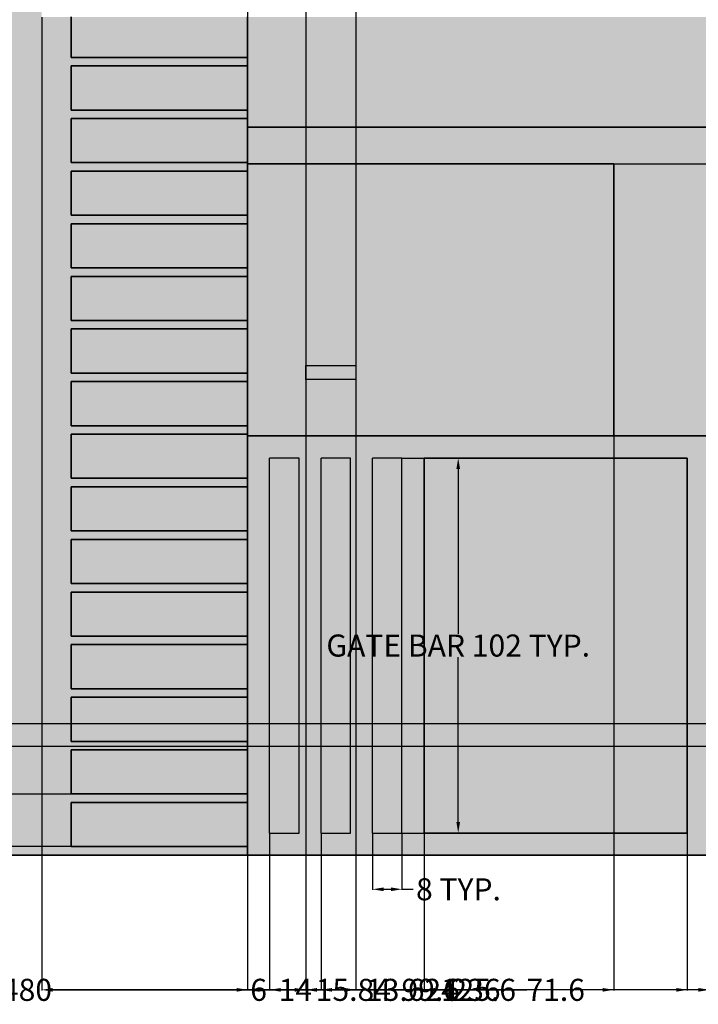
# Model space of a CAD drawing. Units: inches. Extents: x 126 to 726, y 86 to 888.
# Tile 4 of 13: x 424 to 609, y 86 to 354. Entities that reach past the tile are written whole.
import ezdxf

# ---------------------------------------------------------------- set-up
doc = ezdxf.new("R2010")
doc.units = ezdxf.units.IN
doc.header["$MEASUREMENT"] = 0
for name, color, linetype, lineweight in [('A-ANNO-DIMS', 2, 'Continuous', 18), ('A-DOOR', 3, 'Continuous', 25), ('A-ELEV', 7, 'Continuous', 35), ('A-ELEV-GATE', 7, 'Continuous', 25), ('A-ELEV-PATT', 8, 'Continuous', 13)]:
    doc.layers.add(name, color=color, linetype=linetype, lineweight=lineweight)
doc.styles.get("Standard").update_dxf_attribs({"font": 'arial.ttf'})
doc.dimstyles.get("Standard").update_dxf_attribs({"dimtxt": 6, "dimasz": 3, "dimexe": 0.18, "dimexo": 0.0625, "dimgap": 0.09, "dimtad": 0, "dimtih": 1, "dimtoh": 1, "dimdec": 0, "dimzin": 0, "dimdsep": 46, "dimlunit": 3, "dimtxsty": 'Standard', "dimcen": 0.09, "dimadec": 0, "dimazin": 0, "dimtfac": 1, "dimtdec": 0, "dimtofl": 0, "dimtmove": 0, "dimatfit": 3, "dimfxl": 1, "dimtolj": 1, "dimtzin": 0, "dimarcsym": 0})

# ---------------------------------------------------------------- blocks, each defined once
blk = doc.blocks.new('FACADE-STRIP')
for p, q in [((0, 0), (0, 12)), ((0, 12), (48, 12)), ((0, 0), (48, 0))]:
    blk.add_line(p, q)
blk = doc.blocks.new('GATE-BAR')
for p, q in [((0, 0), (0, 102)), ((8, 102), (0, 102)), ((8, 0), (8, 102)), ((0, 0), (8, 0))]:
    blk.add_line(p, q)
blk = doc.blocks.new('*D7')
at = {"layer": 'A-ANNO-DIMS', "color": 0, "lineweight": -2, "transparency": 16777216}
for p, q in [((528.04, 235.04), (543.45, 235.04)), ((543.27, 232.04), (543.27, 187.23)), ((543.27, 136.04), (543.27, 180.85)), ((528.04, 133.04), (543.45, 133.04))]:
    blk.add_line(p, q, dxfattribs=at)
at = {"layer": 'A-ANNO-DIMS', "color": 0, "transparency": 16777216}
for points in [[(542.77, 232.04), (543.77, 232.04), (543.27, 235.04)], [(542.77, 136.04), (543.77, 136.04), (543.27, 133.04)]]:
    blk.add_solid(points, dxfattribs=at)
at = {"layer": 'Defpoints', "color": 0, "transparency": 16777216}
for p in [(527.97, 235.04), (543.27, 235.04), (527.97, 133.04)]:
    blk.add_point(p, dxfattribs=at)
at = {"layer": 'A-ANNO-DIMS', "color": 0, "transparency": 16777216, "insert": (543.27, 184.04), "char_height": 6, "attachment_point": 5}
blk.add_mtext('\\A1;GATE BAR 102 TYP.', dxfattribs=at)
blk = doc.blocks.new('*D8')
at = {"layer": 'A-ANNO-DIMS', "color": 0, "lineweight": -2, "transparency": 16777216}
for p, q in [((519.97, 132.98), (519.97, 117.56)), ((527.97, 132.98), (527.97, 117.56)), ((522.97, 117.74), (524.97, 117.74)), ((527.97, 117.74), (530.97, 117.74))]:
    blk.add_line(p, q, dxfattribs=at)
at = {"layer": 'A-ANNO-DIMS', "color": 0, "transparency": 16777216}
for points in [[(522.97, 118.24), (522.97, 117.24), (519.97, 117.74)], [(524.97, 118.24), (524.97, 117.24), (527.97, 117.74)]]:
    blk.add_solid(points, dxfattribs=at)
at = {"layer": 'Defpoints', "color": 0, "transparency": 16777216}
for p in [(519.97, 133.04), (527.97, 133.04), (527.97, 117.74)]:
    blk.add_point(p, dxfattribs=at)
at = {"layer": 'A-ANNO-DIMS', "color": 0, "transparency": 16777216, "insert": (543.34, 117.74), "char_height": 6, "attachment_point": 5}
blk.add_mtext('\\A1;8 TYP.', dxfattribs=at)
blk = doc.blocks.new('*D13')
at = {"layer": 'A-ANNO-DIMS', "color": 0, "lineweight": -2, "transparency": 16777216}
for p, q in [((665.97, 642.98), (665.97, 90.21)), ((185.97, 126.98), (185.97, 90.21)), ((188.97, 90.39), (419.15, 90.39)), ((662.97, 90.39), (432.8, 90.39))]:
    blk.add_line(p, q, dxfattribs=at)
at = {"layer": 'A-ANNO-DIMS', "color": 0, "transparency": 16777216}
for points in [[(188.97, 90.89), (188.97, 89.89), (185.97, 90.39)], [(662.97, 90.89), (662.97, 89.89), (665.97, 90.39)]]:
    blk.add_solid(points, dxfattribs=at)
at = {"layer": 'Defpoints', "color": 0, "transparency": 16777216}
for p in [(665.97, 643.04), (185.97, 127.04), (665.97, 90.39)]:
    blk.add_point(p, dxfattribs=at)
at = {"layer": 'A-ANNO-DIMS', "color": 0, "transparency": 16777216, "insert": (425.97, 90.39), "char_height": 6, "attachment_point": 5}
blk.add_mtext('\\A1;480', dxfattribs=at)
blk = doc.blocks.new('*D18')
at = {"layer": 'A-ANNO-DIMS', "color": 0, "lineweight": -2, "transparency": 16777216}
for p, q in [((431.28, 395.58), (149.14, 395.58)), ((149.32, 392.58), (149.32, 264.47)), ((149.32, 130.04), (149.32, 258.16)), ((185.91, 127.04), (149.14, 127.04))]:
    blk.add_line(p, q, dxfattribs=at)
at = {"layer": 'A-ANNO-DIMS', "color": 0, "transparency": 16777216}
for points in [[(148.82, 392.58), (149.82, 392.58), (149.32, 395.58)], [(148.82, 130.04), (149.82, 130.04), (149.32, 127.04)]]:
    blk.add_solid(points, dxfattribs=at)
at = {"layer": 'Defpoints', "color": 0, "transparency": 16777216}
for p in [(149.32, 395.58), (431.34, 395.58), (185.97, 127.04)]:
    blk.add_point(p, dxfattribs=at)
at = {"layer": 'A-ANNO-DIMS', "color": 0, "transparency": 16777216, "insert": (149.32, 261.31), "char_height": 6, "attachment_point": 5}
blk.add_mtext('\\A1;268.54', dxfattribs=at)
blk = doc.blocks.new('*D40')
at = {"layer": 'A-ANNO-DIMS', "color": 0, "lineweight": -2, "transparency": 16777216}
for p, q in [((702.62, 165.86), (702.62, 168.86)), ((702.62, 168.86), (705.62, 168.86)), ((346.12, 162.86), (702.8, 162.86)), ((363.55, 156.71), (702.8, 156.71)), ((702.62, 153.71), (702.62, 150.71))]:
    blk.add_line(p, q, dxfattribs=at)
at = {"layer": 'A-ANNO-DIMS', "color": 0, "transparency": 16777216}
for points in [[(702.12, 165.86), (703.12, 165.86), (702.62, 162.86)], [(702.12, 153.71), (703.12, 153.71), (702.62, 156.71)]]:
    blk.add_solid(points, dxfattribs=at)
at = {"layer": 'Defpoints', "color": 0, "transparency": 16777216}
for p in [(346.06, 162.86), (702.62, 162.86), (363.49, 156.71)]:
    blk.add_point(p, dxfattribs=at)
at = {"layer": 'A-ANNO-DIMS', "color": 0, "transparency": 16777216, "insert": (715.86, 168.86), "char_height": 6, "attachment_point": 5}
blk.add_mtext('\\A1;6.149', dxfattribs=at)
blk = doc.blocks.new('*D42')
at = {"layer": 'A-ANNO-DIMS', "color": 0, "lineweight": -2, "transparency": 16777216}
for p, q in [((429.97, 354.98), (429.97, 90.21)), ((665.97, 354.98), (665.97, 90.21)), ((432.97, 90.39), (541.21, 90.39)), ((662.97, 90.39), (554.74, 90.39))]:
    blk.add_line(p, q, dxfattribs=at)
at = {"layer": 'A-ANNO-DIMS', "color": 0, "transparency": 16777216}
for points in [[(432.97, 90.89), (432.97, 89.89), (429.97, 90.39)], [(662.97, 90.89), (662.97, 89.89), (665.97, 90.39)]]:
    blk.add_solid(points, dxfattribs=at)
at = {"layer": 'Defpoints', "color": 0, "transparency": 16777216}
for p in [(429.97, 355.04), (665.97, 355.04), (665.97, 90.39)]:
    blk.add_point(p, dxfattribs=at)
at = {"layer": 'A-ANNO-DIMS', "color": 0, "transparency": 16777216, "insert": (547.97, 90.39), "char_height": 6, "attachment_point": 5}
blk.add_mtext('\\A1;236', dxfattribs=at)
blk = doc.blocks.new('*D61')
at = {"layer": 'A-ANNO-DIMS', "color": 0, "lineweight": -2, "transparency": 16777216}
for p, q in [((501.82, 463.42), (501.82, 90.21)), ((515.44, 463.42), (515.44, 90.21)), ((504.82, 90.39), (512.44, 90.39)), ((515.44, 90.39), (518.44, 90.39))]:
    blk.add_line(p, q, dxfattribs=at)
at = {"layer": 'A-ANNO-DIMS', "color": 0, "transparency": 16777216}
for points in [[(504.82, 90.89), (504.82, 89.89), (501.82, 90.39)], [(512.44, 90.89), (512.44, 89.89), (515.44, 90.39)]]:
    blk.add_solid(points, dxfattribs=at)
at = {"layer": 'Defpoints', "color": 0, "transparency": 16777216}
for p in [(501.82, 463.48), (515.44, 463.48), (515.44, 90.39)]:
    blk.add_point(p, dxfattribs=at)
at = {"layer": 'A-ANNO-DIMS', "color": 0, "transparency": 16777216, "insert": (530.69, 90.39), "char_height": 6, "attachment_point": 5}
blk.add_mtext('\\A1;13.624', dxfattribs=at)
blk = doc.blocks.new('*D63')
at = {"layer": 'A-ANNO-DIMS', "color": 0, "lineweight": -2, "transparency": 16777216}
for p, q in [((501.82, 463.42), (501.82, 90.21)), ((485.97, 458.45), (485.97, 90.21)), ((488.97, 90.39), (498.82, 90.39)), ((501.82, 90.39), (504.82, 90.39))]:
    blk.add_line(p, q, dxfattribs=at)
at = {"layer": 'A-ANNO-DIMS', "color": 0, "transparency": 16777216}
for points in [[(488.97, 90.89), (488.97, 89.89), (485.97, 90.39)], [(498.82, 90.89), (498.82, 89.89), (501.82, 90.39)]]:
    blk.add_solid(points, dxfattribs=at)
at = {"layer": 'Defpoints', "color": 0, "transparency": 16777216}
for p in [(501.82, 463.48), (485.97, 458.51), (501.82, 90.39)]:
    blk.add_point(p, dxfattribs=at)
at = {"layer": 'A-ANNO-DIMS', "color": 0, "transparency": 16777216, "insert": (514.74, 90.39), "char_height": 6, "attachment_point": 5}
blk.add_mtext('\\A1;15.84', dxfattribs=at)
blk = doc.blocks.new('*D65')
at = {"layer": 'A-ANNO-DIMS', "color": 0, "lineweight": -2, "transparency": 16777216}
for p, q in [((485.97, 314.98), (485.97, 90.21)), ((585.58, 314.98), (585.58, 90.21)), ((488.97, 90.39), (527.9, 90.39)), ((582.58, 90.39), (543.66, 90.39))]:
    blk.add_line(p, q, dxfattribs=at)
at = {"layer": 'A-ANNO-DIMS', "color": 0, "transparency": 16777216}
for points in [[(488.97, 90.89), (488.97, 89.89), (485.97, 90.39)], [(582.58, 90.89), (582.58, 89.89), (585.58, 90.39)]]:
    blk.add_solid(points, dxfattribs=at)
at = {"layer": 'Defpoints', "color": 0, "transparency": 16777216}
for p in [(485.97, 315.04), (585.58, 315.04), (585.58, 90.39)]:
    blk.add_point(p, dxfattribs=at)
at = {"layer": 'A-ANNO-DIMS', "color": 0, "transparency": 16777216, "insert": (535.78, 90.39), "char_height": 6, "attachment_point": 5}
blk.add_mtext('\\A1;99.6', dxfattribs=at)
blk = doc.blocks.new('*D66')
at = {"layer": 'A-ANNO-DIMS', "color": 0, "lineweight": -2, "transparency": 16777216}
for p, q in [((585.644259, 315.042369), (702.804909, 315.042369)), ((702.624909, 312.042369), (702.624909, 281.132369)), ((702.624909, 244.042369), (702.624909, 274.952369)), ((585.644259, 241.042369), (702.804909, 241.042369))]:
    blk.add_line(p, q, dxfattribs=at)
at = {"layer": 'A-ANNO-DIMS', "color": 0, "transparency": 16777216}
for points in [[(702.124909, 312.042369), (703.124909, 312.042369), (702.624909, 315.042369)], [(702.124909, 244.042369), (703.124909, 244.042369), (702.624909, 241.042369)]]:
    blk.add_solid(points, dxfattribs=at)
at = {"layer": 'Defpoints', "color": 0, "transparency": 16777216}
for p in [(585.581759, 315.042369), (702.624909, 315.042369), (585.581759, 241.042369)]:
    blk.add_point(p, dxfattribs=at)
at = {"layer": 'A-ANNO-DIMS', "color": 0, "transparency": 16777216, "insert": (702.624909, 278.042369), "char_height": 6, "attachment_point": 5}
blk.add_mtext('\\A1;74', dxfattribs=at)
blk = doc.blocks.new('*D67')
at = {"layer": 'A-ANNO-DIMS', "color": 0, "lineweight": -2, "transparency": 16777216}
for p, q in [((702.624909, 328.042369), (702.624909, 331.042369)), ((631.186514, 325.042369), (702.804909, 325.042369)), ((585.644259, 315.042369), (702.804909, 315.042369)), ((702.624909, 312.042369), (702.624909, 309.042369))]:
    blk.add_line(p, q, dxfattribs=at)
at = {"layer": 'A-ANNO-DIMS', "color": 0, "transparency": 16777216}
for points in [[(702.124909, 328.042369), (703.124909, 328.042369), (702.624909, 325.042369)], [(702.124909, 312.042369), (703.124909, 312.042369), (702.624909, 315.042369)]]:
    blk.add_solid(points, dxfattribs=at)
at = {"layer": 'Defpoints', "color": 0, "transparency": 16777216}
for p in [(631.124014, 325.042369), (702.624909, 325.042369), (585.581759, 315.042369)]:
    blk.add_point(p, dxfattribs=at)
at = {"layer": 'A-ANNO-DIMS', "color": 0, "transparency": 16777216, "insert": (702.624909, 320.042369), "char_height": 6, "attachment_point": 5}
blk.add_mtext('\\A1;10', dxfattribs=at)
blk = doc.blocks.new('*D69')
at = {"layer": 'A-ANNO-DIMS', "color": 0, "lineweight": -2, "transparency": 16777216}
for p, q in [((485.97, 126.98), (485.97, 90.21)), ((611.58, 126.98), (611.58, 90.21)), ((488.97, 90.39), (538.85, 90.39)), ((608.58, 90.39), (558.71, 90.39))]:
    blk.add_line(p, q, dxfattribs=at)
at = {"layer": 'A-ANNO-DIMS', "color": 0, "transparency": 16777216}
for points in [[(488.97, 90.89), (488.97, 89.89), (485.97, 90.39)], [(608.58, 90.89), (608.58, 89.89), (611.58, 90.39)]]:
    blk.add_solid(points, dxfattribs=at)
at = {"layer": 'Defpoints', "color": 0, "transparency": 16777216}
for p in [(485.97, 127.04), (611.58, 127.04), (611.58, 90.39)]:
    blk.add_point(p, dxfattribs=at)
at = {"layer": 'A-ANNO-DIMS', "color": 0, "transparency": 16777216, "insert": (548.78, 90.39), "char_height": 6, "attachment_point": 5}
blk.add_mtext('\\A1;125.6', dxfattribs=at)
blk = doc.blocks.new('*D71')
at = {"layer": 'A-ANNO-DIMS', "color": 0, "lineweight": -2, "transparency": 16777216}
for p, q in [((491.974909, 132.979869), (491.974909, 90.212369)), ((485.974909, 129.290979), (485.974909, 90.212369)), ((482.974909, 90.392369), (479.974909, 90.392369)), ((494.974909, 90.392369), (497.974909, 90.392369))]:
    blk.add_line(p, q, dxfattribs=at)
at = {"layer": 'A-ANNO-DIMS', "color": 0, "transparency": 16777216}
for points in [[(482.974909, 90.892369), (482.974909, 89.892369), (485.974909, 90.392369)], [(494.974909, 90.892369), (494.974909, 89.892369), (491.974909, 90.392369)]]:
    blk.add_solid(points, dxfattribs=at)
at = {"layer": 'Defpoints', "color": 0, "transparency": 16777216}
for p in [(491.974909, 133.042369), (485.974909, 129.353479), (491.974909, 90.392369)]:
    blk.add_point(p, dxfattribs=at)
at = {"layer": 'A-ANNO-DIMS', "color": 0, "transparency": 16777216, "insert": (488.974909, 90.392369), "char_height": 6, "attachment_point": 5}
blk.add_mtext('\\A1;6', dxfattribs=at)
blk = doc.blocks.new('*D72')
at = {"layer": 'A-ANNO-DIMS', "color": 0, "lineweight": -2, "transparency": 16777216}
for p, q in [((491.974909, 132.979869), (491.974909, 90.212369)), ((505.974909, 132.979869), (505.974909, 90.212369)), ((488.974909, 90.392369), (485.974909, 90.392369)), ((508.974909, 90.392369), (511.974909, 90.392369))]:
    blk.add_line(p, q, dxfattribs=at)
at = {"layer": 'A-ANNO-DIMS', "color": 0, "transparency": 16777216}
for points in [[(488.974909, 90.892369), (488.974909, 89.892369), (491.974909, 90.392369)], [(508.974909, 90.892369), (508.974909, 89.892369), (505.974909, 90.392369)]]:
    blk.add_solid(points, dxfattribs=at)
at = {"layer": 'Defpoints', "color": 0, "transparency": 16777216}
for p in [(491.974909, 133.042369), (505.974909, 133.042369), (505.974909, 90.392369)]:
    blk.add_point(p, dxfattribs=at)
at = {"layer": 'A-ANNO-DIMS', "color": 0, "transparency": 16777216, "insert": (498.974909, 90.392369), "char_height": 6, "attachment_point": 5}
blk.add_mtext('\\A1;14', dxfattribs=at)
blk = doc.blocks.new('*D73')
at = {"layer": 'A-ANNO-DIMS', "color": 0, "lineweight": -2, "transparency": 16777216}
for p, q in [((533.97, 132.98), (533.97, 90.21)), ((605.58, 132.98), (605.58, 90.21)), ((536.97, 90.39), (561.92, 90.39)), ((602.58, 90.39), (577.63, 90.39))]:
    blk.add_line(p, q, dxfattribs=at)
at = {"layer": 'A-ANNO-DIMS', "color": 0, "transparency": 16777216}
for points in [[(536.97, 90.89), (536.97, 89.89), (533.97, 90.39)], [(602.58, 90.89), (602.58, 89.89), (605.58, 90.39)]]:
    blk.add_solid(points, dxfattribs=at)
at = {"layer": 'Defpoints', "color": 0, "transparency": 16777216}
for p in [(533.97, 133.04), (605.58, 133.04), (605.58, 90.39)]:
    blk.add_point(p, dxfattribs=at)
at = {"layer": 'A-ANNO-DIMS', "color": 0, "transparency": 16777216, "insert": (569.78, 90.39), "char_height": 6, "attachment_point": 5}
blk.add_mtext('\\A1;71.6', dxfattribs=at)
blk = doc.blocks.new('*D79')
at = {"layer": 'A-ANNO-DIMS', "color": 0, "lineweight": -2, "transparency": 16777216}
for p, q in [((149.32, 132.35), (149.32, 135.35)), ((437.91, 129.35), (149.14, 129.35)), ((485.91, 127.04), (149.14, 127.04)), ((149.32, 124.04), (149.32, 121.04)), ((149.32, 121.04), (146.32, 121.04))]:
    blk.add_line(p, q, dxfattribs=at)
at = {"layer": 'A-ANNO-DIMS', "color": 0, "transparency": 16777216}
for points in [[(148.82, 132.35), (149.82, 132.35), (149.32, 129.35)], [(148.82, 124.04), (149.82, 124.04), (149.32, 127.04)]]:
    blk.add_solid(points, dxfattribs=at)
at = {"layer": 'Defpoints', "color": 0, "transparency": 16777216}
for p in [(437.97, 129.35), (149.32, 127.04), (485.97, 127.04)]:
    blk.add_point(p, dxfattribs=at)
at = {"layer": 'A-ANNO-DIMS', "color": 0, "transparency": 16777216, "insert": (136.64, 121.04), "char_height": 6, "attachment_point": 5}
blk.add_mtext('\\A1;2.311', dxfattribs=at)
blk = doc.blocks.new('*D80')
at = {"layer": 'A-ANNO-DIMS', "color": 0, "lineweight": -2, "transparency": 16777216}
for p, q in [((437.91, 143.66), (149.14, 143.66)), ((149.32, 140.66), (149.32, 139.66)), ((149.32, 132.35), (149.32, 133.35)), ((437.91, 129.35), (149.14, 129.35))]:
    blk.add_line(p, q, dxfattribs=at)
at = {"layer": 'A-ANNO-DIMS', "color": 0, "transparency": 16777216}
for points in [[(148.82, 140.66), (149.82, 140.66), (149.32, 143.66)], [(148.82, 132.35), (149.82, 132.35), (149.32, 129.35)]]:
    blk.add_solid(points, dxfattribs=at)
at = {"layer": 'Defpoints', "color": 0, "transparency": 16777216}
for p in [(149.32, 143.66), (437.97, 143.66), (437.97, 129.35)]:
    blk.add_point(p, dxfattribs=at)
at = {"layer": 'A-ANNO-DIMS', "color": 0, "transparency": 16777216, "insert": (149.32, 136.51), "char_height": 6, "attachment_point": 5}
blk.add_mtext('\\A1;14.31', dxfattribs=at)

msp = doc.modelspace()

# ---------------------------------------------------------------- hatches: boundary and pattern name
at = {"layer": 'A-ELEV-PATT'}
h = msp.add_hatch(color=256, dxfattribs=at)
h.dxf.hatch_style = 1
h.paths.add_polyline_path([(437.9749, 499.1312), (485.9749, 499.1312), (485.9749, 501.4423), (437.9749, 501.4423), (437.9749, 513.4423), (485.9749, 513.4423), (485.9749, 515.7534), (437.9749, 515.7534), (437.9749, 527.7534), (485.9749, 527.7534), (485.9749, 530.0646), (437.9749, 530.0646), (437.9749, 542.0646), (485.9749, 542.0646), (485.9749, 544.3757), (437.9749, 544.3757), (437.9749, 556.3757), (485.9749, 556.3757), (485.9749, 558.6868), (437.9749, 558.6868), (437.9749, 570.6868), (485.9749, 570.6868), (485.9749, 572.9979), (437.9749, 572.9979), (437.9749, 584.9979), (485.9749, 584.9979), (485.9749, 587.309), (437.9749, 587.309), (437.9749, 595.0424), (429.9749, 595.0424), (429.9749, 607.0424), (437.9749, 607.0424), (437.9749, 615.9312), (437.9749, 630.2423), (437.9749, 642.2423), (485.9749, 642.2423), (485.9749, 644.5534), (437.9749, 644.5534), (437.9749, 656.5534), (485.9749, 656.5534), (485.9749, 658.8645), (437.9749, 658.8645), (437.9749, 670.8645), (485.9749, 670.8645), (485.9749, 673.1757), (437.9749, 673.1757), (437.9749, 685.1757), (485.9749, 685.1757), (485.9749, 687.4868), (437.9749, 687.4868), (437.9749, 699.4868), (485.9749, 699.4868), (485.9749, 701.7979), (437.9749, 701.7979), (437.9749, 713.7979), (485.9749, 713.7979), (485.9749, 716.109), (437.9749, 716.109), (437.9749, 728.109), (485.9749, 728.109), (485.9749, 730.4201), (437.9749, 730.4201), (437.9749, 742.4201), (485.9749, 742.4201), (485.9749, 744.7312), (437.9749, 744.7312), (437.9749, 756.7312), (485.9749, 756.7312), (485.9749, 759.0423), (437.9749, 759.0423), (437.9749, 771.0423), (485.9749, 771.0423), (485.9749, 773.3534), (437.9749, 773.3534), (437.9749, 785.3534), (485.9749, 785.3534), (485.9749, 787.6645), (437.9749, 787.6645), (437.9749, 799.6645), (485.9749, 799.6645), (485.9749, 801.9756), (437.9749, 801.9756), (437.9749, 811.2868), (485.9749, 811.2868), (485.9749, 813.9756), (437.9749, 813.9756), (437.9749, 825.9756), (485.9749, 825.9756), (485.9749, 835.0424), (233.9749, 835.0424), (233.9749, 606.5846), (185.9749, 606.5846), (185.9749, 597.5846), (233.9749, 597.5846), (233.9749, 585.5846), (185.9749, 585.5846), (185.9749, 580.5846), (233.9749, 580.5846), (233.9749, 568.5846), (185.9749, 568.5846), (185.9749, 563.5846), (431.3386, 563.5846), (431.3386, 545.5846), (233.9749, 545.5846), (233.9749, 413.5846), (431.3386, 413.5846), (431.3386, 395.5846), (185.9749, 395.5846), (185.9749, 386.5846), (233.9749, 386.5846), (233.9749, 374.5846), (185.9749, 374.5846), (185.9749, 369.5846), (233.9749, 369.5846), (233.9749, 357.5846), (185.9749, 357.5846), (185.9749, 352.5846), (233.9749, 352.5846), (233.9749, 340.5846), (185.9749, 340.5846), (185.9749, 331.5846), (233.9749, 331.5846), (233.9749, 127.0424), (485.9749, 127.0424), (485.9749, 129.3535), (437.9749, 129.3535), (437.9749, 141.3535), (485.9749, 141.3535), (485.9749, 143.6646), (437.9749, 143.6646), (437.9749, 155.6646), (485.9749, 155.6646), (485.9749, 157.9757), (437.9749, 157.9757), (437.9749, 169.9757), (485.9749, 169.9757), (485.9749, 172.2868), (437.9749, 172.2868), (437.9749, 184.2868), (485.9749, 184.2868), (485.9749, 186.5979), (437.9749, 186.5979), (437.9749, 198.5979), (485.9749, 198.5979), (485.9749, 200.909), (437.9749, 200.909), (437.9749, 212.909), (485.9749, 212.909), (485.9749, 215.2201), (437.9749, 215.2201), (437.9749, 227.2201), (485.9749, 227.2201), (485.9749, 229.5312), (437.9749, 229.5312), (437.9749, 241.5312), (485.9749, 241.5312), (485.9749, 243.8424), (437.9749, 243.8424), (437.9749, 255.8424), (485.9749, 255.8424), (485.9749, 258.1535), (437.9749, 258.1535), (437.9749, 270.1535), (485.9749, 270.1535), (485.9749, 272.4646), (437.9749, 272.4646), (437.9749, 284.4646), (485.9749, 284.4646), (485.9749, 286.7757), (437.9749, 286.7757), (437.9749, 298.7757), (485.9749, 298.7757), (485.9749, 301.0868), (437.9749, 301.0868), (437.9749, 313.0868), (485.9749, 313.0868), (485.9749, 315.3979), (437.9749, 315.3979), (437.9749, 327.3979), (485.9749, 327.3979), (485.9749, 329.709), (437.9749, 329.709), (437.9749, 341.709), (485.9749, 341.709), (485.9749, 344.0201), (437.9749, 344.0201), (437.9749, 355.0424), (429.9749, 355.0424), (429.9749, 367.0424), (437.9749, 367.0424), (437.9749, 372.6423), (437.9749, 386.9535), (437.9749, 401.2646), (437.9749, 413.2646), (485.9749, 413.2646), (485.9749, 415.5757), (437.9749, 415.5757), (437.9749, 427.5757), (485.9749, 427.5757), (485.9749, 429.8868), (437.9749, 429.8868), (437.9749, 441.8868), (485.9749, 441.8868), (485.9749, 444.1979), (437.9749, 444.1979), (437.9749, 456.1979), (485.9749, 456.1979), (485.9749, 458.509), (437.9749, 458.509), (437.9749, 470.509), (485.9749, 470.509), (485.9749, 472.8201), (437.9749, 472.8201), (437.9749, 484.8201), (485.9749, 484.8201), (485.9749, 487.1312), (437.9749, 487.1312)])
h.paths.add_polyline_path([(299.6658, 533.6845), (371.6658, 533.6845), (371.6658, 425.6845), (299.6658, 425.6845)], flags=16)
h.paths.add_polyline_path([(308.6658, 524.6845), (362.6658, 524.6845), (362.6658, 434.6845), (308.6658, 434.6845)], flags=0)
h.paths.add_polyline_path([(317.7956, 603.3211, -0.4129833), (306.8418, 614.321, -0.94403766), (328.769, 615.5845, -0.04423165), (330.7031, 615.4048, -0.89973713), (352.5798, 615.6161, -0.4129833), (363.5336, 604.6162, -0.94403766), (341.6064, 603.3528, -0.04423165), (339.6723, 603.5324, -0.89973713)], flags=16)
h.paths.add_polyline_path([(319.7228, 604.5846, -0.02633223), (319.7726, 605.5306, -0.47905713), (308.8418, 614.321, -1), (326.8418, 614.321, -0.02633223), (326.7919, 613.375, -0.17413188), (332.826, 612.5948, -0.04918553), (332.6526, 614.3527, -1), (350.6526, 614.3527, -0.02633223), (350.6028, 613.4067, -0.47905713), (361.5336, 604.6162, -1), (343.5336, 604.6162, -0.02633223), (343.5834, 605.5622, -0.17413188), (337.5494, 606.3424, -0.04918553), (337.7228, 604.5846, -1)], flags=0)
h.paths.add_polyline_path([(328.769, 355.6561, -0.04423165), (330.7031, 355.4765, -0.89973713), (352.5798, 355.6878, -0.4129833), (363.5336, 344.6879, -0.94403766), (341.6064, 343.4244, -0.04423165), (339.6723, 343.604, -0.89973713), (317.7956, 343.3927, -0.4129833), (306.8418, 354.3926, -0.94403766)], flags=16)
h.paths.add_polyline_path([(326.8418, 354.3926, -0.02633223), (326.7919, 353.4466, -0.17413188), (332.826, 352.6664, -0.04918553), (332.6526, 354.4243, -1), (350.6526, 354.4243, -0.02633223), (350.6028, 353.4783, -0.47905713), (361.5336, 344.6879, -1), (343.5336, 344.6879, -0.02633223), (343.5834, 345.6339, -0.17413188), (337.5494, 346.4141, -0.04918553), (337.7228, 344.6562, -1), (319.7228, 344.6562, -0.02633223), (319.7726, 345.6022, -0.47905713), (308.8418, 354.3926, -1)], flags=0)
h.paths.add_polyline_path([(299.3189, 655.3527), (299.3189, 763.3527), (371.3189, 763.3527), (371.3189, 655.3527)], flags=16)
h.paths.add_polyline_path([(308.3189, 664.3527), (308.3189, 754.3527), (362.3189, 754.3527), (362.3189, 664.3527)], flags=0)
h.paths.add_polyline_path([(299.6658, 303.5875), (371.6658, 303.5875), (371.6658, 195.5875), (299.6658, 195.5875)], flags=16)
h.paths.add_polyline_path([(308.6658, 294.5875), (362.6658, 294.5875), (362.6658, 204.5875), (308.6658, 204.5875)], flags=0)
h.paths.add_polyline_path([(326.3038, 177.3867), (346.055, 177.3867, -0.41421356), (349.055, 174.3867), (349.055, 171.2378), (363.489, 171.2378, -0.41421356), (366.489, 168.2378), (366.489, 159.7133, -0.41421356), (363.489, 156.7133), (343.7379, 156.7133, -0.41421356), (340.7379, 159.7133), (340.7379, 162.8622), (330.5504, 162.8622), (330.5504, 159.7133, -0.41421356), (327.5504, 156.7133), (307.7992, 156.7133, -0.41421356), (304.7992, 159.7133), (304.7992, 168.2378, -0.41421356), (307.7992, 171.2378), (323.3038, 171.2378), (323.3038, 174.3867, -0.41421356)], flags=16)
h.paths.add_polyline_path([(326.3038, 175.3867), (346.055, 175.3867, -0.41421356), (347.055, 174.3867), (347.055, 169.2378), (363.489, 169.2378, -0.41421356), (364.489, 168.2378), (364.489, 159.7133, -0.41421356), (363.489, 158.7133), (343.7379, 158.7133, -0.41421356), (342.7379, 159.7133), (342.7379, 164.8622), (328.5504, 164.8622), (328.5504, 159.7133, -0.41421356), (327.5504, 158.7133), (307.7992, 158.7133, -0.41421356), (306.7992, 159.7133), (306.7992, 168.2378, -0.41421356), (307.7992, 169.2378), (325.3038, 169.2378), (325.3038, 174.3867, -0.41421356)], flags=0)
h = msp.add_hatch(dxfattribs=at)
h.set_pattern_fill('GRAVEL', color=256, scale=40)
h.paths.add_polyline_path([(437.9749, 642.2423), (485.9749, 642.2423), (485.9749, 644.5534), (437.9749, 644.5534), (437.9749, 656.5534), (485.9749, 656.5534), (485.9749, 658.8645), (437.9749, 658.8645), (437.9749, 670.8645), (485.9749, 670.8645), (485.9749, 673.1757), (437.9749, 673.1757), (437.9749, 685.1757), (485.9749, 685.1757), (485.9749, 687.4868), (437.9749, 687.4868), (437.9749, 699.4868), (485.9749, 699.4868), (485.9749, 701.7979), (437.9749, 701.7979), (437.9749, 713.7979), (485.9749, 713.7979), (485.9749, 716.109), (437.9749, 716.109), (437.9749, 728.109), (485.9749, 728.109), (485.9749, 730.4201), (437.9749, 730.4201), (437.9749, 742.4201), (485.9749, 742.4201), (485.9749, 744.7312), (437.9749, 744.7312), (437.9749, 756.7312), (485.9749, 756.7312), (485.9749, 759.0423), (437.9749, 759.0423), (437.9749, 771.0423), (485.9749, 771.0423), (485.9749, 773.3534), (437.9749, 773.3534), (437.9749, 785.3534), (485.9749, 785.3534), (485.9749, 787.6645), (437.9749, 787.6645), (437.9749, 799.6645), (485.9749, 799.6645), (485.9749, 801.9756), (437.9749, 801.9756), (437.9749, 811.2868), (485.9749, 811.2868), (485.9749, 813.9756), (437.9749, 813.9756), (437.9749, 825.9756), (485.9749, 825.9756), (485.9749, 835.0424), (233.9749, 835.0424), (233.9749, 606.5846), (185.9749, 606.5846), (185.9749, 597.5846), (233.9749, 597.5846), (233.9749, 585.5846), (185.9749, 585.5846), (185.9749, 580.5846), (233.9749, 580.5846), (233.9749, 568.5846), (185.9749, 568.5846), (185.9749, 563.5846), (431.3386, 563.5846), (431.3386, 545.5846), (233.9749, 545.5846), (233.9749, 413.5846), (431.3386, 413.5846), (431.3386, 395.5846), (185.9749, 395.5846), (185.9749, 386.5846), (233.9749, 386.5846), (233.9749, 374.5846), (185.9749, 374.5846), (185.9749, 369.5846), (233.9749, 369.5846), (233.9749, 357.5846), (185.9749, 357.5846), (185.9749, 352.5846), (233.9749, 352.5846), (233.9749, 340.5846), (185.9749, 340.5846), (185.9749, 331.5846), (233.9749, 331.5846), (233.9749, 127.0424), (485.9749, 127.0424), (485.9749, 129.3535), (437.9749, 129.3535), (437.9749, 141.3535), (485.9749, 141.3535), (485.9749, 143.6646), (437.9749, 143.6646), (437.9749, 155.6646), (485.9749, 155.6646), (485.9749, 157.9757), (437.9749, 157.9757), (437.9749, 169.9757), (485.9749, 169.9757), (485.9749, 172.2868), (437.9749, 172.2868), (437.9749, 184.2868), (485.9749, 184.2868), (485.9749, 186.5979), (437.9749, 186.5979), (437.9749, 198.5979), (485.9749, 198.5979), (485.9749, 200.909), (437.9749, 200.909), (437.9749, 212.909), (485.9749, 212.909), (485.9749, 215.2201), (437.9749, 215.2201), (437.9749, 227.2201), (485.9749, 227.2201), (485.9749, 229.5312), (437.9749, 229.5312), (437.9749, 241.5312), (485.9749, 241.5312), (485.9749, 243.8424), (437.9749, 243.8424), (437.9749, 255.8424), (485.9749, 255.8424), (485.9749, 258.1535), (437.9749, 258.1535), (437.9749, 270.1535), (485.9749, 270.1535), (485.9749, 272.4646), (437.9749, 272.4646), (437.9749, 284.4646), (485.9749, 284.4646), (485.9749, 286.7757), (437.9749, 286.7757), (437.9749, 298.7757), (485.9749, 298.7757), (485.9749, 301.0868), (437.9749, 301.0868), (437.9749, 313.0868), (485.9749, 313.0868), (485.9749, 315.3979), (437.9749, 315.3979), (437.9749, 327.3979), (485.9749, 327.3979), (485.9749, 329.709), (437.9749, 329.709), (437.9749, 341.709), (485.9749, 341.709), (485.9749, 344.0201), (437.9749, 344.0201), (437.9749, 355.0424), (429.9749, 355.0424), (429.9749, 367.0424), (437.9749, 367.0424), (437.9749, 372.6423), (437.9749, 386.9535), (437.9749, 401.2646), (437.9749, 413.2646), (485.9749, 413.2646), (485.9749, 415.5757), (437.9749, 415.5757), (437.9749, 427.5757), (485.9749, 427.5757), (485.9749, 429.8868), (437.9749, 429.8868), (437.9749, 441.8868), (485.9749, 441.8868), (485.9749, 444.1979), (437.9749, 444.1979), (437.9749, 456.1979), (485.9749, 456.1979), (485.9749, 458.509), (437.9749, 458.509), (437.9749, 470.509), (485.9749, 470.509), (485.9749, 472.8201), (437.9749, 472.8201), (437.9749, 484.8201), (485.9749, 484.8201), (485.9749, 487.1312), (437.9749, 487.1312), (437.9749, 499.1312), (485.9749, 499.1312), (485.9749, 501.4423), (437.9749, 501.4423), (437.9749, 513.4423), (485.9749, 513.4423), (485.9749, 515.7534), (437.9749, 515.7534), (437.9749, 527.7534), (485.9749, 527.7534), (485.9749, 530.0646), (437.9749, 530.0646), (437.9749, 542.0646), (485.9749, 542.0646), (485.9749, 544.3757), (437.9749, 544.3757), (437.9749, 556.3757), (485.9749, 556.3757), (485.9749, 558.6868), (437.9749, 558.6868), (437.9749, 570.6868), (485.9749, 570.6868), (485.9749, 572.9979), (437.9749, 572.9979), (437.9749, 584.9979), (485.9749, 584.9979), (485.9749, 587.309), (437.9749, 587.309), (437.9749, 595.0424), (429.9749, 595.0424), (429.9749, 607.0424), (437.9749, 607.0424), (437.9749, 615.9312), (437.9749, 630.2423)])
h.paths.add_polyline_path([(371.3189, 655.3527), (299.3189, 655.3527), (299.3189, 763.3527), (371.3189, 763.3527)], flags=16)
h.paths.add_polyline_path([(363.5336, 604.6162, -0.94403766), (341.6064, 603.3528, -0.04423165), (339.6723, 603.5324, -0.89973713), (317.7956, 603.3211, -0.4129833), (306.8418, 614.321, -0.94403766), (328.769, 615.5845, -0.04423165), (330.7031, 615.4048, -0.89973713), (352.5798, 615.6161, -0.4129833)], flags=16)
h.paths.add_polyline_path([(361.5336, 604.6162, -1), (343.5336, 604.6162, -0.02633223), (343.5834, 605.5622, -0.17413188), (337.5494, 606.3424, -0.04918553), (337.7228, 604.5846, -1), (319.7228, 604.5846, -0.02633223), (319.7726, 605.5306, -0.47905713), (308.8418, 614.321, -1), (326.8418, 614.321, -0.02633223), (326.7919, 613.375, -0.17413188), (332.826, 612.5948, -0.04918553), (332.6526, 614.3527, -1), (350.6526, 614.3527, -0.02633223), (350.6028, 613.4067, -0.47905713)], flags=0)
h.paths.add_polyline_path([(362.3189, 664.3527), (308.3189, 664.3527), (308.3189, 754.3527), (362.3189, 754.3527)], flags=0)
h.paths.add_polyline_path([(371.6658, 533.6845), (371.6658, 425.6845), (299.6658, 425.6845), (299.6658, 533.6845)], flags=16)
h.paths.add_polyline_path([(362.6658, 524.6845), (362.6658, 434.6845), (308.6658, 434.6845), (308.6658, 524.6845)], flags=0)
h.paths.add_polyline_path([(352.5798, 355.6878, -0.4129833), (363.5336, 344.6879, -0.94403766), (341.6064, 343.4244, -0.04423165), (339.6723, 343.604, -0.89973713), (317.7956, 343.3927, -0.4129833), (306.8418, 354.3926, -0.94403766), (328.769, 355.6561, -0.04423165), (330.7031, 355.4765, -0.89973713)], flags=16)
h.paths.add_polyline_path([(350.6526, 354.4243, -0.02633223), (350.6028, 353.4783, -0.47905713), (361.5336, 344.6879, -1), (343.5336, 344.6879, -0.02633223), (343.5834, 345.6339, -0.17413188), (337.5494, 346.4141, -0.04918553), (337.7228, 344.6562, -1), (319.7228, 344.6562, -0.02633223), (319.7726, 345.6022, -0.47905713), (308.8418, 354.3926, -1), (326.8418, 354.3926, -0.02633223), (326.7919, 353.4466, -0.17413188), (332.826, 352.6664, -0.04918553), (332.6526, 354.4243, -1)], flags=0)
h.paths.add_polyline_path([(371.6658, 303.5875), (371.6658, 195.5875), (299.6658, 195.5875), (299.6658, 303.5875)], flags=16)
h.paths.add_polyline_path([(362.6658, 294.5875), (362.6658, 204.5875), (308.6658, 204.5875), (308.6658, 294.5875)], flags=0)
h.paths.add_polyline_path([(346.055, 177.3867, -0.41421356), (349.055, 174.3867), (349.055, 171.2378), (363.489, 171.2378, -0.41421356), (366.489, 168.2378), (366.489, 159.7133, -0.41421356), (363.489, 156.7133), (343.7379, 156.7133, -0.41421356), (340.7379, 159.7133), (340.7379, 162.8622), (330.5504, 162.8622), (330.5504, 159.7133, -0.41421356), (327.5504, 156.7133), (307.7992, 156.7133, -0.41421356), (304.7992, 159.7133), (304.7992, 168.2378, -0.41421356), (307.7992, 171.2378), (323.3038, 171.2378), (323.3038, 174.3867, -0.41421356), (326.3038, 177.3867)], flags=16)
h.paths.add_polyline_path([(346.055, 175.3867, -0.41421356), (347.055, 174.3867), (347.055, 169.2378), (363.489, 169.2378, -0.41421356), (364.489, 168.2378), (364.489, 159.7133, -0.41421356), (363.489, 158.7133), (343.7379, 158.7133, -0.41421356), (342.7379, 159.7133), (342.7379, 164.8622), (328.5504, 164.8622), (328.5504, 159.7133, -0.41421356), (327.5504, 158.7133), (307.7992, 158.7133, -0.41421356), (306.7992, 159.7133), (306.7992, 168.2378, -0.41421356), (307.7992, 169.2378), (325.3038, 169.2378), (325.3038, 174.3867, -0.41421356), (326.3038, 175.3867)], flags=0)
h = msp.add_hatch(color=256, dxfattribs=at)
h.dxf.hatch_style = 1
h.paths.add_polyline_path([(485.9749, 595.0424), (485.9749, 564.6845), (585.5818, 564.6845), (585.5818, 595.0424)])
h.paths.add_polyline_path([(660.0469, 325.0424), (660.0469, 355.0424), (485.9749, 355.0424), (485.9749, 325.0424)])
h = msp.add_hatch(color=256, dxfattribs=at)
h.dxf.hatch_style = 1
h.paths.add_polyline_path([(515.4403, 260.2201), (501.8163, 260.2201), (501.8163, 256.3808), (515.4403, 256.3808)])
h.paths.add_polyline_path([(515.4403, 467.321), (501.8163, 467.321), (501.8163, 463.4817), (515.4403, 463.4817)])
h = msp.add_hatch(color=256, dxfattribs=at)
h.dxf.hatch_style = 1
h.paths.add_polyline_path([(585.5818, 403.0424), (485.9749, 403.0424), (485.9749, 367.0424), (585.5818, 367.0424)])
h.paths.add_polyline_path([(527.9749, 235.0424), (519.9749, 235.0424), (519.9749, 133.0424), (527.9749, 133.0424)])
h.paths.add_polyline_path([(513.9749, 235.0424), (505.9749, 235.0424), (505.9749, 133.0424), (513.9749, 133.0424)])
h.paths.add_polyline_path([(499.9749, 235.0424), (491.9749, 235.0424), (491.9749, 133.0424), (499.9749, 133.0424)])
h = msp.add_hatch(color=256, dxfattribs=at)
h.dxf.hatch_style = 1
h.paths.add_polyline_path([(485.9749, 129.3535), (485.9749, 141.3535), (437.9749, 141.3535), (437.9749, 129.3535)])
h.paths.add_polyline_path([(437.9749, 155.6646), (437.9749, 143.6646), (485.9749, 143.6646), (485.9749, 155.6646)])
h.paths.add_polyline_path([(485.9749, 157.9757), (485.9749, 169.9757), (437.9749, 169.9757), (437.9749, 157.9757)])
h.paths.add_polyline_path([(485.9749, 172.2868), (485.9749, 184.2868), (437.9749, 184.2868), (437.9749, 172.2868)])
h.paths.add_polyline_path([(485.9749, 186.5979), (485.9749, 198.5979), (437.9749, 198.5979), (437.9749, 186.5979)])
h.paths.add_polyline_path([(485.9749, 200.909), (485.9749, 212.909), (437.9749, 212.909), (437.9749, 200.909)])
h.paths.add_polyline_path([(485.9749, 215.2201), (485.9749, 227.2201), (437.9749, 227.2201), (437.9749, 215.2201)])
h.paths.add_polyline_path([(437.9749, 241.5312), (437.9749, 229.5312), (485.9749, 229.5312), (485.9749, 241.5312)])
h.paths.add_polyline_path([(485.9749, 243.8424), (485.9749, 255.8424), (437.9749, 255.8424), (437.9749, 243.8424)])
h.paths.add_polyline_path([(485.9749, 258.1535), (485.9749, 270.1535), (437.9749, 270.1535), (437.9749, 258.1535)])
h.paths.add_polyline_path([(485.9749, 272.4646), (485.9749, 284.4646), (437.9749, 284.4646), (437.9749, 272.4646)])
h.paths.add_polyline_path([(485.9749, 286.7757), (485.9749, 298.7757), (437.9749, 298.7757), (437.9749, 286.7757)])
h.paths.add_polyline_path([(437.9749, 313.0868), (437.9749, 301.0868), (485.9749, 301.0868), (485.9749, 313.0868)])
h.paths.add_polyline_path([(437.9749, 327.3979), (437.9749, 315.3979), (485.9749, 315.3979), (485.9749, 327.3979)])
h.paths.add_polyline_path([(485.9749, 329.709), (485.9749, 341.709), (437.9749, 341.709), (437.9749, 329.709)])
h.paths.add_polyline_path([(485.9749, 344.0201), (485.9749, 355.0424), (437.9749, 355.0424), (437.9749, 344.0201)])
h.paths.add_polyline_path([(437.9749, 384.6423), (437.9749, 372.6423), (485.9749, 372.6423), (485.9749, 384.6423)])
h.paths.add_polyline_path([(437.9749, 398.9535), (437.9749, 386.9535), (485.9749, 386.9535), (485.9749, 398.9535)])
h = msp.add_hatch(color=256, dxfattribs=at)
h.dxf.hatch_style = 1
h.paths.add_polyline_path([(631.124, 325.0424), (485.9749, 325.0424), (485.9749, 315.0424), (585.5818, 315.0424), (585.5818, 241.0424), (611.5818, 241.0424), (611.5818, 229.0424), (631.124, 229.0424)])
h = msp.add_hatch(color=256, dxfattribs=at)
h.dxf.hatch_style = 1
h.paths.add_polyline_path([(631.124, 325.0424), (585.5818, 325.0424), (585.5818, 241.0424), (611.5818, 241.0424), (611.5818, 229.0424), (631.124, 229.0424)])
h = msp.add_hatch(color=256, dxfattribs=at)
h.dxf.hatch_style = 1
h.paths.add_polyline_path([(585.5818, 315.0424), (485.9749, 315.0424), (485.9749, 241.0424), (585.5818, 241.0424)])
h.paths.add_polyline_path([(515.4403, 260.2201), (515.4403, 256.3808), (501.8163, 256.3808), (501.8163, 260.2201)], flags=16)
h = msp.add_hatch(color=256, dxfattribs=at)
h.dxf.hatch_style = 1
h.paths.add_polyline_path([(611.5818, 241.0424), (485.9749, 241.0424), (485.9749, 127.0424), (611.5818, 127.0424), (611.5818, 229.0424)])
h.paths.add_polyline_path([(505.9749, 235.0424), (513.9749, 235.0424), (513.9749, 133.0424), (505.9749, 133.0424)], flags=16)
h.paths.add_polyline_path([(499.9749, 235.0424), (499.9749, 133.0424), (491.9749, 133.0424), (491.9749, 235.0424)], flags=16)
h.paths.add_polyline_path([(519.9749, 235.0424), (527.9749, 235.0424), (527.9749, 133.0424), (519.9749, 133.0424)], flags=16)
h.paths.add_polyline_path([(533.9749, 235.0424), (605.5818, 235.0424), (605.5818, 133.0424), (533.9749, 133.0424)], flags=16)
h = msp.add_hatch(color=256, dxfattribs=at)
h.dxf.hatch_style = 1
h.paths.add_polyline_path([(605.5818, 235.0424), (533.9749, 235.0424), (533.9749, 133.0424), (605.5818, 133.0424)])

# ---------------------------------------------------------------- linework, layer by layer
at = {"layer": 'A-DOOR'}
msp.add_lwpolyline([(501.8163, 260.2201), (515.4403, 260.2201), (515.4403, 256.3808), (501.8163, 256.3808)], close=True, dxfattribs=at)
at = {"layer": 'A-ELEV'}
for p, q in [((437.9749, 344.0201), (437.9749, 355.0424)), ((485.9749, 127.0424), (485.9749, 355.0424)), ((437.9749, 344.0201), (485.9749, 344.0201)), ((660.0469, 325.0424), (485.9749, 325.0424)), ((585.5818, 315.0424), (485.9749, 315.0424)), ((585.5818, 315.0424), (585.5818, 241.0424)), ((611.5818, 241.0424), (485.9749, 241.0424)), ((605.5818, 235.0424), (533.9749, 235.0424)), ((533.9749, 133.0424), (533.9749, 235.0424)), ((605.5818, 235.0424), (605.5818, 133.0424)), ((533.9749, 133.0424), (605.5818, 133.0424)), ((185.9749, 127.0424), (660.0469, 127.0424)), ((437.9749, 127.0424), (485.9749, 127.0424))]:
    msp.add_line(p, q, dxfattribs=at)

# ---------------------------------------------------------------- block references
for p in [(437.975, 329.7085), (437.975, 315.3974), (437.975, 301.0863), (437.975, 286.7752), (437.975, 272.4641), (437.975, 258.153), (437.975, 243.8419), (437.975, 229.5308), (437.975, 215.2197), (437.975, 200.9085), (437.975, 186.5974), (437.975, 172.2863), (437.975, 157.9752), (437.975, 143.6641), (437.975, 129.353)]:
    msp.add_blockref('FACADE-STRIP', p, dxfattribs=at)
at = {"layer": 'A-ELEV-GATE'}
for p in [(491.975, 133.042), (505.975, 133.042), (519.975, 133.042)]:
    msp.add_blockref('GATE-BAR', p, dxfattribs=at)

# ---------------------------------------------------------------- dimensions: what is measured, and where the dimension line sits
at = {"layer": 'A-ANNO-DIMS'}
for base, p1, p2, override, picture, middle in [((665.9749, 90.3924), (185.9749, 127.0424), (665.9749, 643.0424), {"dimdec": 0, "dimlfac": 1, "dimrnd": 0, "dimzin": 0, "dimdsep": 46, "dimlunit": 2}, '*D13', (425.9749, 90.3924)), ((501.8163, 90.3924), (485.9749, 458.509), (501.8163, 463.4817), {"dimdec": 2, "dimlfac": 1, "dimrnd": 0, "dimzin": 0, "dimdsep": 46, "dimlunit": 2}, '*D63', (514.7351, 90.3924)), ((515.4403, 90.3924), (501.8163, 463.4817), (515.4403, 463.4817), {"dimdec": 3, "dimlfac": 1, "dimrnd": 0, "dimzin": 0, "dimdsep": 46, "dimlunit": 2}, '*D61', (530.6899, 90.3924)), ((665.9749, 90.3924), (429.9749, 355.0424), (665.9749, 355.0424), {"dimdec": 0, "dimlfac": 1, "dimrnd": 0, "dimzin": 0, "dimdsep": 46, "dimlunit": 2}, '*D42', (547.9749, 90.3924)), ((585.5818, 90.3924), (485.9749, 315.0424), (585.5818, 315.0424), {"dimdec": 1, "dimlfac": 1, "dimrnd": 0, "dimzin": 0, "dimdsep": 46, "dimlunit": 2}, '*D65', (535.7783, 90.3924)), ((491.9749, 90.3924), (485.9749, 129.3535), (491.9749, 133.0424), {"dimdec": 0, "dimlfac": 1, "dimrnd": 0, "dimzin": 0, "dimdsep": 46, "dimlunit": 2}, '*D71', (488.9749, 90.3924)), ((505.9749, 90.3924), (491.9749, 133.0424), (505.9749, 133.0424), {"dimdec": 0, "dimlfac": 1, "dimrnd": 0, "dimzin": 0, "dimdsep": 46, "dimlunit": 2}, '*D72', (498.9749, 90.3924)), ((605.5818, 90.3924), (533.9749, 133.0424), (605.5818, 133.0424), {"dimdec": 1, "dimlfac": 1, "dimrnd": 0, "dimzin": 0, "dimdsep": 46, "dimlunit": 2}, '*D73', (569.7783, 90.3924)), ((611.5818, 90.3924), (485.9749, 127.0424), (611.5818, 127.0424), {"dimdec": 1, "dimlfac": 1, "dimrnd": 0, "dimzin": 0, "dimdsep": 46, "dimlunit": 2}, '*D69', (548.7783, 90.3924))]:
    dim = msp.add_linear_dim(base=base, p1=p1, p2=p2, dimstyle='Standard', override=override, dxfattribs=at)
    dim.commit()
    dim.dimension.update_dxf_attribs({"geometry": picture, "text_midpoint": middle})
for base, p1, p2, override, picture, middle in [((149.3249, 395.5846), (185.9749, 127.0424), (431.3386, 395.5846), {"dimdec": 2, "dimlfac": 1, "dimrnd": 0, "dimzin": 0, "dimdsep": 46, "dimlunit": 2}, '*D18', (149.3249, 261.3135)), ((702.6249, 325.0424), (585.5818, 315.0424), (631.124, 325.0424), {"dimdec": 0, "dimlfac": 1, "dimrnd": 0, "dimzin": 0, "dimdsep": 46, "dimlunit": 2}, '*D67', (702.6249, 320.0424)), ((702.6249, 315.0424), (585.5818, 241.0424), (585.5818, 315.0424), {"dimdec": 0, "dimlfac": 1, "dimrnd": 0, "dimzin": 0, "dimdsep": 46, "dimlunit": 2}, '*D66', (702.6249, 278.0424)), ((702.6249, 162.8622), (363.489, 156.7133), (346.055, 162.8622), {"dimdec": 3, "dimlfac": 1, "dimrnd": 0, "dimzin": 0, "dimdsep": 46, "dimlunit": 2}, '*D40', (715.8609, 168.8622)), ((149.3249, 143.6646), (437.9749, 129.3535), (437.9749, 143.6646), {"dimdec": 2, "dimlfac": 1, "dimrnd": 0, "dimzin": 0, "dimdsep": 46, "dimlunit": 2}, '*D80', (149.3249, 136.509)), ((149.3249, 127.0424), (437.9749, 129.3535), (485.9749, 127.0424), {"dimdec": 3, "dimlfac": 1, "dimrnd": 0, "dimzin": 0, "dimdsep": 46, "dimlunit": 2}, '*D79', (136.6394, 121.0424))]:
    dim = msp.add_linear_dim(base=base, p1=p1, p2=p2, angle=90, dimstyle='Standard', override=override, dxfattribs=at)
    dim.commit()
    dim.dimension.update_dxf_attribs({"geometry": picture, "text_midpoint": middle})
dim = msp.add_linear_dim(base=(543.2749, 235.0424), p1=(527.9749, 133.0424), p2=(527.9749, 235.0424), angle=90, text='GATE BAR <> TYP.', dimstyle='Standard', override={"dimdec": 0, "dimlfac": 1, "dimrnd": 0, "dimzin": 0, "dimdsep": 46, "dimlunit": 2}, dxfattribs=at)
dim.commit()
dim.dimension.update_dxf_attribs({"geometry": '*D7', "text_midpoint": (543.2749, 184.0424)})
dim = msp.add_linear_dim(base=(527.9749, 117.7424), p1=(519.9749, 133.0424), p2=(527.9749, 133.0424), text='<> TYP.', dimstyle='Standard', override={"dimdec": 0, "dimlfac": 1, "dimrnd": 0, "dimzin": 0, "dimdsep": 46, "dimlunit": 2}, dxfattribs=at)
dim.commit()
dim.dimension.update_dxf_attribs({"geometry": '*D8', "text_midpoint": (543.3412, 117.7424)})

doc.saveas('drawing.dxf')
